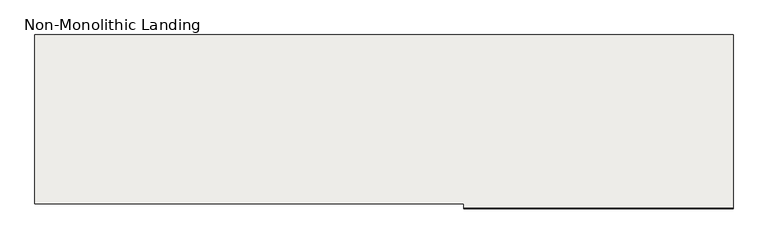
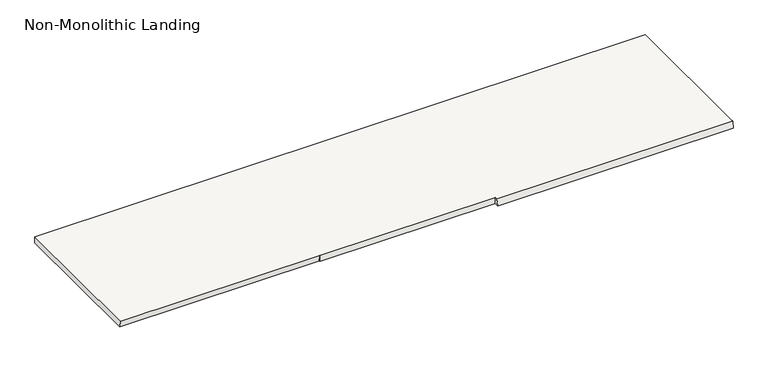
"""IFC4 building model written with IfcOpenShell, lengths in millimetres: slab geometry, Non-Monolithic Landing."""

from ifc_helpers import new_model, si_unit, origin, place, context, project, spatial, faceted_brep, source, transform, mapped, element, save


def non_monolithic_landing_b96f42b5(model_context):
    return source(origin(), model_context, "Body", "Brep", [
        faceted_brep([(466.2714992, 10367.1981148, 1217.3913043), (466.2714992, 10360.0106148, 1167.3913043), (2255.6816567, 10360.0106148, 1167.3913043), (2255.6816567, 10367.1981148, 1217.3913043), (-866.6164824, 10392.1981148, 1217.3913043), (466.2714992, 10392.1981148, 1217.3913043), (2255.6816567, 10392.1981148, 1217.3913043), (2255.6816567, 11513.685068, 1217.3913043), (-2381.5205334, 11513.685068, 1217.3913043), (-2381.5205334, 10392.1981148, 1217.3913043), (466.2714992, 10392.1981148, 1167.3913043), (-866.6164824, 10392.1981148, 1167.3913043), (-866.6164824, 10399.3856148, 1167.3913043), (-2381.5205334, 10399.3856148, 1167.3913043), (-2381.5205334, 11513.685068, 1167.3913043), (2255.6816567, 11513.685068, 1167.3913043), (2255.6816567, 10392.1981148, 1167.3913043)], [[[0, 1, 2, 3]], [[4, 5, 0, 3, 6, 7, 8, 9]], [[10, 11, 12, 13, 14, 15, 16, 2, 1]], [[5, 4, 11, 10]], [[0, 5, 10, 1]], [[6, 3, 2, 16]], [[7, 6, 16, 15]], [[8, 7, 15, 14]], [[9, 8, 14, 13]], [[4, 12, 11]], [[12, 4, 9, 13]]]),
    ])


if __name__ == "__main__":
    model = new_model("IFC4")
    model_context = context("Model", 3, world=origin())
    ifc_project = project(units=[si_unit("LENGTHUNIT", "METRE", prefix="MILLI")], contexts=[model_context])
    site = spatial("IfcSite", under=ifc_project)
    building = spatial("IfcBuilding", under=site)
    placement = place(None, origin())
    non_monolithic_landing_shape = non_monolithic_landing_b96f42b5(model_context)
    element("IfcSlab", 1, ObjectType="Non-Monolithic Landing", at=placement, inside=building, context=model_context, shape_type="MappedRepresentation", body=[
        mapped(non_monolithic_landing_shape, transform((0.0, 0.0, 0.0), x_axis=(1.0, 0.0, 0.0), y_axis=(0.0, 1.0, 0.0), z_axis=(0.0, 0.0, 1.0))),
    ])
    save(model, "model.ifc")
